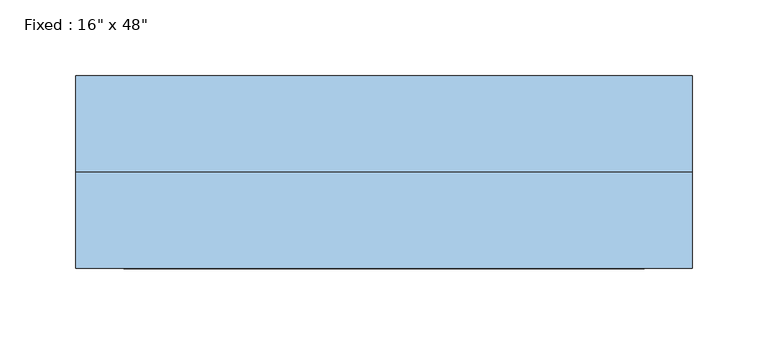
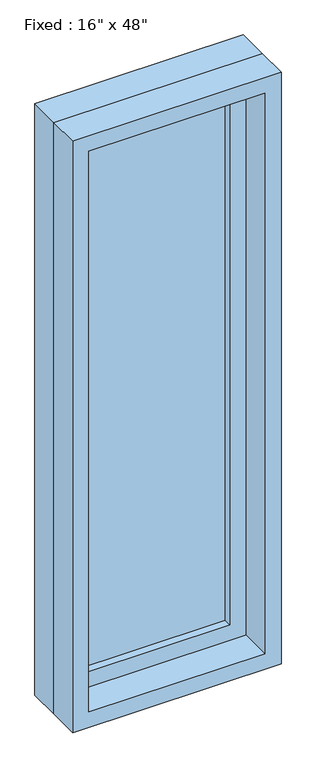
"""IFC4 building model written with IfcOpenShell, lengths in millimetres: window geometry."""

from ifc_helpers import new_model, si_unit, frame, origin, place, context, project, spatial, polyline, outline, extrude, source, transform, mapped, element, save


def window_f83fec05(model_context):
    return source(origin(), model_context, "Body", "SweptSolid", [
        extrude(outline(polyline([(101.6, 15.875), (-177.8, 15.875), (-177.8, 28.575), (101.6, 28.575), (101.6, 15.875)])), frame((0.0, 0.0, 977.9), z_axis=(0.0, 0.0, 1.0), x_axis=(1.0, 0.0, 0.0)), (0.0, 0.0, 1.0), 1092.2),
        extrude(outline(polyline([(2114.55, -222.25), (933.45, -222.25), (933.45, 146.05), (2114.55, 146.05), (2114.55, -222.25)]), holes=[polyline([(2070.1, -177.8), (2070.1, 101.6), (977.9, 101.6), (977.9, -177.8), (2070.1, -177.8)])]), frame((0.0, 0.0, 0.0), z_axis=(0.0, 1.0, 0.0), x_axis=(0.0, 0.0, 1.0)), (0.0, 0.0, 1.0), 44.45),
        extrude(outline(polyline([(2133.6, -241.3), (914.4, -241.3), (914.4, 165.1), (2133.6, 165.1), (2133.6, -241.3)]), holes=[polyline([(2101.85, -209.55), (2101.85, 133.35), (946.15, 133.35), (946.15, -209.55), (2101.85, -209.55)])]), frame((0.0, -63.5, 0.0), z_axis=(0.0, 1.0, 0.0), x_axis=(0.0, 0.0, 1.0)), (0.0, 0.0, 1.0), 63.5),
        extrude(outline(polyline([(2133.6, 165.1), (2133.6, -241.3), (914.4, -241.3), (914.4, 165.1), (2133.6, 165.1)]), holes=[polyline([(2114.55, 146.05), (933.45, 146.05), (933.45, -222.25), (2114.55, -222.25), (2114.55, 146.05)])]), frame((0.0, 0.0, 0.0), z_axis=(0.0, 1.0, 0.0), x_axis=(0.0, 0.0, 1.0)), (0.0, 0.0, 1.0), 63.5),
    ])


if __name__ == "__main__":
    model = new_model("IFC4")
    model_context = context("Model", 3, world=origin())
    ifc_project = project(units=[si_unit("LENGTHUNIT", "METRE", prefix="MILLI")], contexts=[model_context])
    site = spatial("IfcSite", under=ifc_project)
    building = spatial("IfcBuilding", under=site)
    placement = place(None, origin())
    window_shape = window_f83fec05(model_context)
    element("IfcWindow", 1, ObjectType="Fixed : 16\" x 48\"", at=placement, inside=building, context=model_context, shape_type="MappedRepresentation", body=[
        mapped(window_shape, transform((0.0, 0.0, 0.0), x_axis=(1.0, 0.0, 0.0), y_axis=(0.0, 1.0, 0.0), z_axis=(0.0, 0.0, 1.0))),
    ])
    save(model, "model.ifc")

# Revit data of these elements
# Type "Fixed : 16\" x 48\""
#   Type Mark = "5"
#   Construction Type Id = "GSP4R"
#   Assembly Code = "B2020100"
#   Analytic Construction = "1/8 in Pilkington single glazing"
#   Visual Light Transmittance = 0.9
#   Solar Heat Gain Coefficient = 0.78
#   Heat Transfer Coefficient (U) = 0.6496 BTU/(h·ft²·°F)
#   Height = 4' - 0"
#   Default Sill Height = 3' - 0"
#   Width = 1' - 4"
#   Window Inset = 0' - 0 3/4"
#   Define Thermal Properties by = 1
#   Glass Pane Material = Glass
#   Sash Material = Sash
#   Wall Closure = (empty or 0)
# Element 1 (IfcWindow, "Fixed : 16\" x 48\"")
#   Materials on its faces: "Sash", "Glass"
# Materials
#   "Glass": class "Glass", colour RGB 0 128 192, transparency 0.75, Description = "Soda Lime Glass", Cost = 0
#   "Sash": class "Wood", colour RGB 224 178 126, transparency 0
